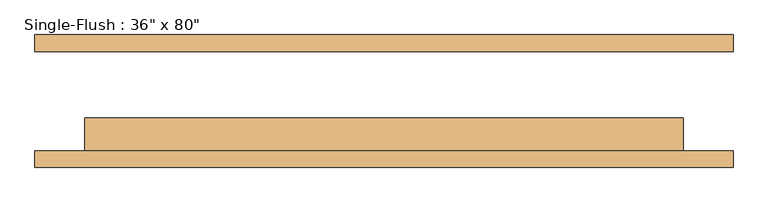
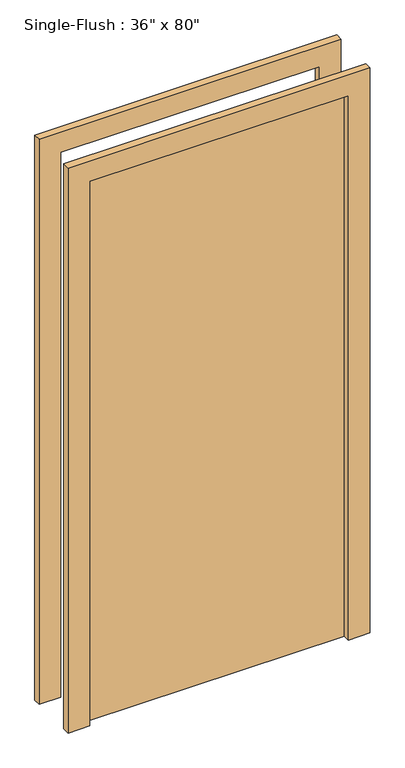
"""IFC4 building model written with IfcOpenShell, lengths in millimetres: door geometry."""

from ifc_helpers import new_model, si_unit, frame, origin, origin_with_axes, place, context, project, spatial, polyline, outline, extrude, source, transform, mapped, element, save


def door_2b0b55a0(model_context):
    return source(origin(), model_context, "Body", "SweptSolid", [
        extrude(outline(polyline([(2108.2, -533.4), (0.0, -533.4), (0.0, -457.2), (2032.0, -457.2), (2032.0, 457.2), (0.0, 457.2), (0.0, 533.4), (2108.2, 533.4), (2108.2, -533.4)])), frame((0.0, -101.6, 0.0), z_axis=(0.0, 1.0, 0.0), x_axis=(0.0, 0.0, 1.0)), (0.0, 0.0, 1.0), 25.4),
        extrude(outline(polyline([(2108.2, 533.4), (2108.2, -533.4), (0.0, -533.4), (0.0, -457.2), (2032.0, -457.2), (2032.0, 457.2), (0.0, 457.2), (0.0, 533.4), (2108.2, 533.4)])), frame((0.0, 76.2, 0.0), z_axis=(0.0, 1.0, 0.0), x_axis=(0.0, 0.0, 1.0)), (0.0, 0.0, 1.0), 25.4),
        extrude(outline(polyline([(457.2, -25.4), (457.2, -76.2), (-457.2, -76.2), (-457.2, -25.4), (457.2, -25.4)])), origin_with_axes(), (0.0, 0.0, 1.0), 2032.0),
    ])


if __name__ == "__main__":
    model = new_model("IFC4")
    model_context = context("Model", 3, world=origin())
    ifc_project = project(units=[si_unit("LENGTHUNIT", "METRE", prefix="MILLI")], contexts=[model_context])
    site = spatial("IfcSite", under=ifc_project)
    building = spatial("IfcBuilding", under=site)
    placement = place(None, origin())
    door_shape = door_2b0b55a0(model_context)
    element("IfcDoor", 1, ObjectType="Single-Flush : 36\" x 80\"", at=placement, inside=building, context=model_context, shape_type="MappedRepresentation", body=[
        mapped(door_shape, transform((0.0, 0.0, 0.0), x_axis=(1.0, 0.0, 0.0), y_axis=(0.0, 1.0, 0.0), z_axis=(0.0, 0.0, 1.0))),
    ])
    save(model, "model.ifc")

# Revit data of these elements
# Type "Single-Flush : 36\" x 80\""
#   Type Mark = "6"
#   Construction Type Id = "MDOOR"
#   Assembly Code = "C1020"
#   Analytic Construction = "Metal"
#   Thickness = 0' - 2"
#   Heat Transfer Coefficient (U) = 0.651978 BTU/(h·ft²·°F)
#   Height = 6' - 8"
#   Trim Projection Ext = 0' - 1"
#   Trim Projection Int = 0' - 1"
#   Trim Width = 0' - 3"
#   Width = 3' - 0"
#   Define Thermal Properties by = 1
#   Define Thermal Properties by = 1
#   Door Material = Door - Panel
#   Frame Material = Door - Frame
#   Visual Light Transmittance = 0
#   Solar Heat Gain Coefficient = 0
#   Function = (empty or 0)
#   Wall Closure = (empty or 0)
# Element 1 (IfcDoor, "Single-Flush : 36\" x 80\"")
#   Materials on its faces: "Door - Frame", "Door - Panel"
# Materials
#   "Door - Panel": class "Wood", colour RGB 210 159 95, transparency 0, Cost = 0
#   "Door - Frame": colour RGB 118 70 51, transparency 0, Cost = 0
